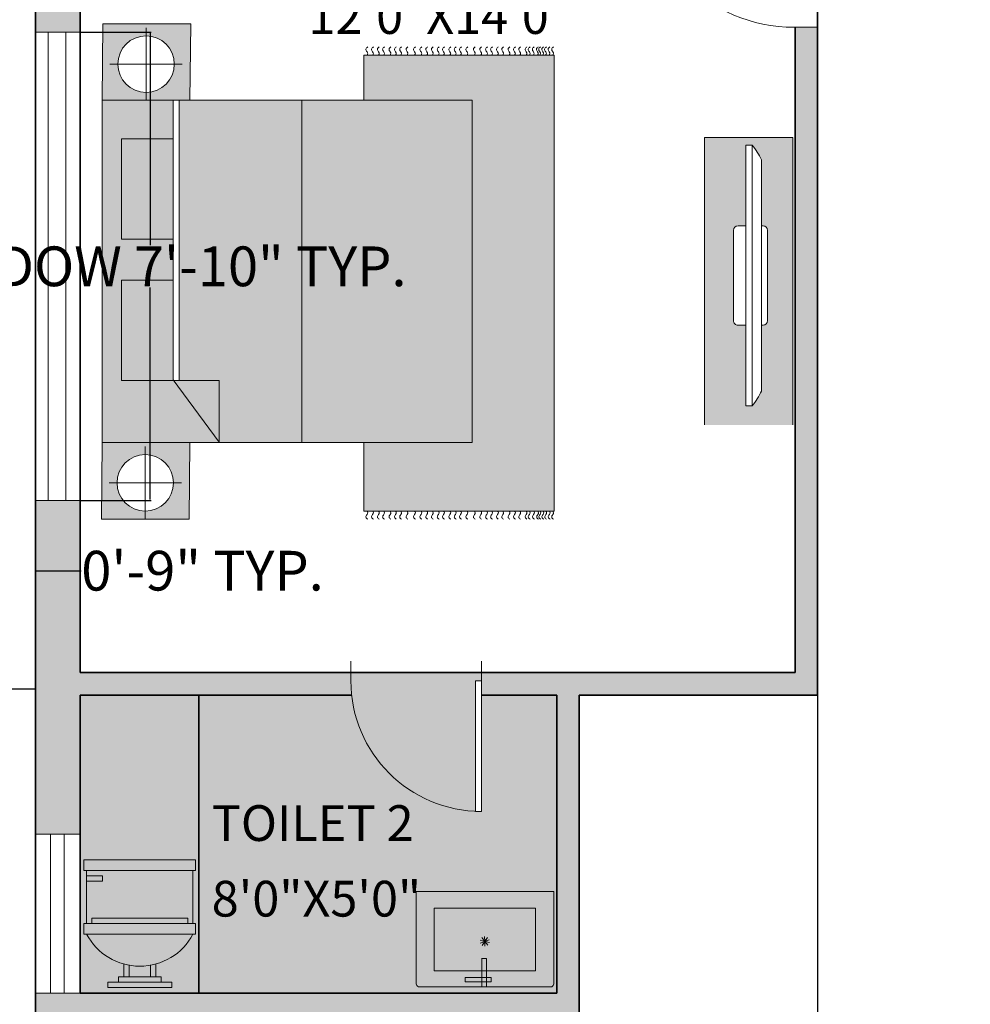
# Model space of a CAD drawing. Units: inches. Extents: x 853 to 1550, y 485 to 1596.
# Tile 4 of 18: x 979 to 1170, y 1010 to 1208. Entities that reach past the tile are written whole.
import ezdxf

# ---------------------------------------------------------------- set-up
doc = ezdxf.new("R2010")
doc.units = ezdxf.units.IN
doc.header["$MEASUREMENT"] = 0
for name, color, linetype, lineweight in [('A-ANNO-DIMS', 2, 'Continuous', 18), ('A-AREA-IDEN', 250, 'Continuous', 18), ('A-DOOR', 4, 'Continuous', 18), ('A-FLOR-CASE', 32, 'Continuous', 25), ('A-FLOR-FIXT', 8, 'Continuous', 18), ('A-WALL-PATT', 250, 'Continuous', 13), ('furniture', 250, 'Continuous', 18), ('walls', 250, 'Continuous', 35), ('windows', 4, 'Continuous', 18)]:
    doc.layers.add(name, color=color, linetype=linetype, lineweight=lineweight)
for name, color, linetype, lineweight, true_color in [('A-FIXT-PATT', 9, 'Continuous', 13, 0xc7c8ca), ('A-FLOR-TILE-PATT', 141, 'Continuous', 13, 0xadddf7), ('A-FURN-PATT', 254, 'Continuous', 13, 0xfeeab9)]:
    doc.layers.add(name, color=color, linetype=linetype, lineweight=lineweight, true_color=true_color)
doc.styles.get("Standard").update_dxf_attribs({"font": 'arial.ttf'})
doc.dimstyles.get("Standard").update_dxf_attribs({"dimtxt": 8, "dimasz": 0.18, "dimexe": 0.18, "dimexo": 0.0625, "dimgap": 0.09, "dimtad": 0, "dimtih": 1, "dimtoh": 1, "dimzin": 0, "dimdsep": 46, "dimlunit": 3, "dimtxsty": 'Standard', "dimcen": 0.09, "dimadec": 0, "dimazin": 0, "dimtfac": 1, "dimtofl": 0, "dimtmove": 0, "dimatfit": 3, "dimfxl": 1, "dimtolj": 1, "dimtzin": 0, "dimarcsym": 0})

# ---------------------------------------------------------------- blocks, each defined once
blk = doc.blocks.new('CARPET')
at = {"layer": 'furniture'}
for p, q in [((-51.53, -98.11), (-51.53, -55.12)), ((-51.53, -55.12), (-41.27, -55.12)), ((36, -55.12), (51.55, -55.12)), ((51.55, -55.12), (51.55, -98.11)), ((51.55, -98.11), (-51.53, -98.11))]:
    blk.add_line(p, q, dxfattribs=at)
for points, knots in [([(-53.37, -55.99), (-53.22, -55.8), (-52.9, -55.41), (-52.34, -55.8), (-51.89, -56.08), (-51.65, -55.91), (-51.53, -55.83)], [0, 0, 0, 0, 0.653278, 1.290138, 1.740457, 2.114451, 2.114451, 2.114451, 2.114451]), ([(53.37, -55.99), (53.22, -55.8), (52.9, -55.41), (52.34, -55.8), (51.89, -56.08), (51.65, -55.91), (51.53, -55.83)], [0, 0, 0, 0, 0.653278, 1.290138, 1.740457, 2.114451, 2.114451, 2.114451, 2.114451]), ([(-53.37, -57.26), (-53.22, -57.07), (-52.9, -56.67), (-52.34, -57.07), (-51.89, -57.35), (-51.65, -57.17), (-51.53, -57.1)], [0, 0, 0, 0, 0.653278, 1.290138, 1.740457, 2.114451, 2.114451, 2.114451, 2.114451]), ([(53.37, -57.26), (53.22, -57.07), (52.9, -56.67), (52.34, -57.07), (51.89, -57.35), (51.65, -57.17), (51.53, -57.1)], [0, 0, 0, 0, 0.653278, 1.290138, 1.740457, 2.114451, 2.114451, 2.114451, 2.114451]), ([(-53.37, -58.59), (-53.22, -58.4), (-52.9, -58.01), (-52.34, -58.4), (-51.89, -58.68), (-51.65, -58.5), (-51.53, -58.43)], [0, 0, 0, 0, 0.653278, 1.290138, 1.740457, 2.114451, 2.114451, 2.114451, 2.114451]), ([(-53.37, -59.78), (-53.22, -59.58), (-52.9, -59.19), (-52.34, -59.58), (-51.89, -59.86), (-51.65, -59.69), (-51.53, -59.61)], [0, 0, 0, 0, 0.653278, 1.290138, 1.740457, 2.114451, 2.114451, 2.114451, 2.114451]), ([(53.37, -58.59), (53.22, -58.4), (52.9, -58.01), (52.34, -58.4), (51.89, -58.68), (51.65, -58.5), (51.53, -58.43)], [0, 0, 0, 0, 0.653278, 1.290138, 1.740457, 2.114451, 2.114451, 2.114451, 2.114451]), ([(53.37, -59.78), (53.22, -59.58), (52.9, -59.19), (52.34, -59.58), (51.89, -59.86), (51.65, -59.69), (51.53, -59.61)], [0, 0, 0, 0, 0.653278, 1.290138, 1.740457, 2.114451, 2.114451, 2.114451, 2.114451]), ([(-53.37, -61.22), (-53.22, -61.02), (-52.9, -60.63), (-52.34, -61.02), (-51.89, -61.3), (-51.65, -61.13), (-51.53, -61.05)], [0, 0, 0, 0, 0.653278, 1.290138, 1.740457, 2.114451, 2.114451, 2.114451, 2.114451]), ([(-53.37, -62.44), (-53.22, -62.25), (-52.9, -61.86), (-52.34, -62.25), (-51.89, -62.53), (-51.65, -62.36), (-51.53, -62.28)], [0, 0, 0, 0, 0.653278, 1.290138, 1.740457, 2.114451, 2.114451, 2.114451, 2.114451]), ([(53.37, -61.22), (53.22, -61.02), (52.9, -60.63), (52.34, -61.02), (51.89, -61.3), (51.65, -61.13), (51.53, -61.05)], [0, 0, 0, 0, 0.653278, 1.290138, 1.740457, 2.114451, 2.114451, 2.114451, 2.114451]), ([(53.37, -62.44), (53.22, -62.25), (52.9, -61.86), (52.34, -62.25), (51.89, -62.53), (51.65, -62.36), (51.53, -62.28)], [0, 0, 0, 0, 0.653278, 1.290138, 1.740457, 2.114451, 2.114451, 2.114451, 2.114451]), ([(-53.37, -63.63), (-53.22, -63.43), (-52.9, -63.04), (-52.34, -63.43), (-51.89, -63.72), (-51.65, -63.54), (-51.53, -63.46)], [0, 0, 0, 0, 0.653278, 1.290138, 1.740457, 2.114451, 2.114451, 2.114451, 2.114451]), ([(53.37, -63.63), (53.22, -63.43), (52.9, -63.04), (52.34, -63.43), (51.89, -63.72), (51.65, -63.54), (51.53, -63.46)], [0, 0, 0, 0, 0.653278, 1.290138, 1.740457, 2.114451, 2.114451, 2.114451, 2.114451]), ([(-53.37, -65.07), (-53.22, -64.87), (-52.9, -64.48), (-52.34, -64.87), (-51.89, -65.15), (-51.65, -64.98), (-51.53, -64.9)], [0, 0, 0, 0, 0.653278, 1.290138, 1.740457, 2.114451, 2.114451, 2.114451, 2.114451]), ([(-53.37, -66.76), (-53.22, -66.56), (-52.9, -66.17), (-52.34, -66.56), (-51.89, -66.84), (-51.65, -66.67), (-51.53, -66.59)], [0, 0, 0, 0, 0.653278, 1.290138, 1.740457, 2.114451, 2.114451, 2.114451, 2.114451]), ([(53.37, -65.07), (53.22, -64.87), (52.9, -64.48), (52.34, -64.87), (51.89, -65.15), (51.65, -64.98), (51.53, -64.9)], [0, 0, 0, 0, 0.653278, 1.290138, 1.740457, 2.114451, 2.114451, 2.114451, 2.114451]), ([(53.37, -66.76), (53.22, -66.56), (52.9, -66.17), (52.34, -66.56), (51.89, -66.84), (51.65, -66.67), (51.53, -66.59)], [0, 0, 0, 0, 0.653278, 1.290138, 1.740457, 2.114451, 2.114451, 2.114451, 2.114451]), ([(-53.37, -68.2), (-53.22, -68), (-52.9, -67.61), (-52.34, -68), (-51.89, -68.28), (-51.65, -68.11), (-51.53, -68.03)], [0, 0, 0, 0, 0.653278, 1.290138, 1.740457, 2.114451, 2.114451, 2.114451, 2.114451]), ([(53.37, -68.2), (53.22, -68), (52.9, -67.61), (52.34, -68), (51.89, -68.28), (51.65, -68.11), (51.53, -68.03)], [0, 0, 0, 0, 0.653278, 1.290138, 1.740457, 2.114451, 2.114451, 2.114451, 2.114451]), ([(-53.37, -69.53), (-53.22, -69.33), (-52.9, -68.94), (-52.34, -69.33), (-51.89, -69.61), (-51.65, -69.44), (-51.53, -69.36)], [0, 0, 0, 0, 0.653278, 1.290138, 1.740457, 2.114451, 2.114451, 2.114451, 2.114451]), ([(-53.37, -70.79), (-53.22, -70.6), (-52.9, -70.21), (-52.34, -70.6), (-51.89, -70.88), (-51.65, -70.7), (-51.53, -70.63)], [0, 0, 0, 0, 0.653278, 1.290138, 1.740457, 2.114451, 2.114451, 2.114451, 2.114451]), ([(53.37, -69.53), (53.22, -69.33), (52.9, -68.94), (52.34, -69.33), (51.89, -69.61), (51.65, -69.44), (51.53, -69.36)], [0, 0, 0, 0, 0.653278, 1.290138, 1.740457, 2.114451, 2.114451, 2.114451, 2.114451]), ([(53.37, -70.79), (53.22, -70.6), (52.9, -70.21), (52.34, -70.6), (51.89, -70.88), (51.65, -70.7), (51.53, -70.63)], [0, 0, 0, 0, 0.653278, 1.290138, 1.740457, 2.114451, 2.114451, 2.114451, 2.114451]), ([(-53.37, -72.12), (-53.22, -71.93), (-52.9, -71.54), (-52.34, -71.93), (-51.89, -72.21), (-51.65, -72.04), (-51.53, -71.96)], [0, 0, 0, 0, 0.653278, 1.290138, 1.740457, 2.114451, 2.114451, 2.114451, 2.114451]), ([(-53.37, -73.31), (-53.22, -73.11), (-52.9, -72.72), (-52.34, -73.11), (-51.89, -73.4), (-51.65, -73.22), (-51.53, -73.14)], [0, 0, 0, 0, 0.653278, 1.290138, 1.740457, 2.114451, 2.114451, 2.114451, 2.114451]), ([(53.37, -72.12), (53.22, -71.93), (52.9, -71.54), (52.34, -71.93), (51.89, -72.21), (51.65, -72.04), (51.53, -71.96)], [0, 0, 0, 0, 0.653278, 1.290138, 1.740457, 2.114451, 2.114451, 2.114451, 2.114451]), ([(53.37, -73.31), (53.22, -73.11), (52.9, -72.72), (52.34, -73.11), (51.89, -73.4), (51.65, -73.22), (51.53, -73.14)], [0, 0, 0, 0, 0.653278, 1.290138, 1.740457, 2.114451, 2.114451, 2.114451, 2.114451]), ([(-53.37, -74.75), (-53.22, -74.55), (-52.9, -74.16), (-52.34, -74.55), (-51.89, -74.83), (-51.65, -74.66), (-51.53, -74.58)], [0, 0, 0, 0, 0.653278, 1.290138, 1.740457, 2.114451, 2.114451, 2.114451, 2.114451]), ([(-53.37, -75.98), (-53.22, -75.78), (-52.9, -75.39), (-52.34, -75.78), (-51.89, -76.06), (-51.65, -75.89), (-51.53, -75.81)], [0, 0, 0, 0, 0.653278, 1.290138, 1.740457, 2.114451, 2.114451, 2.114451, 2.114451]), ([(53.37, -74.75), (53.22, -74.55), (52.9, -74.16), (52.34, -74.55), (51.89, -74.83), (51.65, -74.66), (51.53, -74.58)], [0, 0, 0, 0, 0.653278, 1.290138, 1.740457, 2.114451, 2.114451, 2.114451, 2.114451]), ([(53.37, -75.98), (53.22, -75.78), (52.9, -75.39), (52.34, -75.78), (51.89, -76.06), (51.65, -75.89), (51.53, -75.81)], [0, 0, 0, 0, 0.653278, 1.290138, 1.740457, 2.114451, 2.114451, 2.114451, 2.114451]), ([(-53.37, -77.16), (-53.22, -76.96), (-52.9, -76.57), (-52.34, -76.96), (-51.89, -77.25), (-51.65, -77.07), (-51.53, -76.99)], [0, 0, 0, 0, 0.653278, 1.290138, 1.740457, 2.114451, 2.114451, 2.114451, 2.114451]), ([(53.37, -77.16), (53.22, -76.96), (52.9, -76.57), (52.34, -76.96), (51.89, -77.25), (51.65, -77.07), (51.53, -76.99)], [0, 0, 0, 0, 0.653278, 1.290138, 1.740457, 2.114451, 2.114451, 2.114451, 2.114451]), ([(-53.37, -78.6), (-53.22, -78.4), (-52.9, -78.01), (-52.34, -78.4), (-51.89, -78.68), (-51.65, -78.51), (-51.53, -78.43)], [0, 0, 0, 0, 0.653278, 1.290138, 1.740457, 2.114451, 2.114451, 2.114451, 2.114451]), ([(-53.37, -80.29), (-53.22, -80.09), (-52.9, -79.7), (-52.34, -80.09), (-51.89, -80.37), (-51.65, -80.2), (-51.53, -80.12)], [0, 0, 0, 0, 0.653278, 1.290138, 1.740457, 2.114451, 2.114451, 2.114451, 2.114451]), ([(53.37, -78.6), (53.22, -78.4), (52.9, -78.01), (52.34, -78.4), (51.89, -78.68), (51.65, -78.51), (51.53, -78.43)], [0, 0, 0, 0, 0.653278, 1.290138, 1.740457, 2.114451, 2.114451, 2.114451, 2.114451]), ([(53.37, -80.29), (53.22, -80.09), (52.9, -79.7), (52.34, -80.09), (51.89, -80.37), (51.65, -80.2), (51.53, -80.12)], [0, 0, 0, 0, 0.653278, 1.290138, 1.740457, 2.114451, 2.114451, 2.114451, 2.114451]), ([(-53.37, -81.73), (-53.22, -81.53), (-52.9, -81.14), (-52.34, -81.53), (-51.89, -81.81), (-51.65, -81.64), (-51.53, -81.56)], [0, 0, 0, 0, 0.653278, 1.290138, 1.740457, 2.114451, 2.114451, 2.114451, 2.114451]), ([(53.37, -81.73), (53.22, -81.53), (52.9, -81.14), (52.34, -81.53), (51.89, -81.81), (51.65, -81.64), (51.53, -81.56)], [0, 0, 0, 0, 0.653278, 1.290138, 1.740457, 2.114451, 2.114451, 2.114451, 2.114451]), ([(-53.37, -83.06), (-53.22, -82.86), (-52.9, -82.47), (-52.34, -82.86), (-51.89, -83.14), (-51.65, -82.97), (-51.53, -82.89)], [0, 0, 0, 0, 0.653278, 1.290138, 1.740457, 2.114451, 2.114451, 2.114451, 2.114451]), ([(-53.37, -84.18), (-53.22, -83.99), (-52.9, -83.6), (-52.34, -83.99), (-51.89, -84.27), (-51.65, -84.09), (-51.53, -84.02)], [0, 0, 0, 0, 0.653278, 1.290138, 1.740457, 2.114451, 2.114451, 2.114451, 2.114451]), ([(53.37, -83.06), (53.22, -82.86), (52.9, -82.47), (52.34, -82.86), (51.89, -83.14), (51.65, -82.97), (51.53, -82.89)], [0, 0, 0, 0, 0.653278, 1.290138, 1.740457, 2.114451, 2.114451, 2.114451, 2.114451]), ([(53.37, -84.18), (53.22, -83.99), (52.9, -83.6), (52.34, -83.99), (51.89, -84.27), (51.65, -84.09), (51.53, -84.02)], [0, 0, 0, 0, 0.653278, 1.290138, 1.740457, 2.114451, 2.114451, 2.114451, 2.114451]), ([(-53.37, -85.51), (-53.22, -85.32), (-52.9, -84.93), (-52.34, -85.32), (-51.89, -85.6), (-51.65, -85.42), (-51.53, -85.35)], [0, 0, 0, 0, 0.653278, 1.290138, 1.740457, 2.114451, 2.114451, 2.114451, 2.114451]), ([(-53.37, -86.7), (-53.22, -86.5), (-52.9, -86.11), (-52.34, -86.5), (-51.89, -86.78), (-51.65, -86.61), (-51.53, -86.53)], [0, 0, 0, 0, 0.653278, 1.290138, 1.740457, 2.114451, 2.114451, 2.114451, 2.114451]), ([(53.37, -85.51), (53.22, -85.32), (52.9, -84.93), (52.34, -85.32), (51.89, -85.6), (51.65, -85.42), (51.53, -85.35)], [0, 0, 0, 0, 0.653278, 1.290138, 1.740457, 2.114451, 2.114451, 2.114451, 2.114451]), ([(53.37, -86.7), (53.22, -86.5), (52.9, -86.11), (52.34, -86.5), (51.89, -86.78), (51.65, -86.61), (51.53, -86.53)], [0, 0, 0, 0, 0.653278, 1.290138, 1.740457, 2.114451, 2.114451, 2.114451, 2.114451]), ([(-53.37, -88.14), (-53.22, -87.94), (-52.9, -87.55), (-52.34, -87.94), (-51.89, -88.22), (-51.65, -88.05), (-51.53, -87.97)], [0, 0, 0, 0, 0.653278, 1.290138, 1.740457, 2.114451, 2.114451, 2.114451, 2.114451]), ([(-53.37, -89.36), (-53.22, -89.17), (-52.9, -88.78), (-52.34, -89.17), (-51.89, -89.45), (-51.65, -89.28), (-51.53, -89.2)], [0, 0, 0, 0, 0.653278, 1.290138, 1.740457, 2.114451, 2.114451, 2.114451, 2.114451]), ([(53.37, -88.14), (53.22, -87.94), (52.9, -87.55), (52.34, -87.94), (51.89, -88.22), (51.65, -88.05), (51.53, -87.97)], [0, 0, 0, 0, 0.653278, 1.290138, 1.740457, 2.114451, 2.114451, 2.114451, 2.114451]), ([(53.37, -89.36), (53.22, -89.17), (52.9, -88.78), (52.34, -89.17), (51.89, -89.45), (51.65, -89.28), (51.53, -89.2)], [0, 0, 0, 0, 0.653278, 1.290138, 1.740457, 2.114451, 2.114451, 2.114451, 2.114451]), ([(-53.37, -90.55), (-53.22, -90.35), (-52.9, -89.96), (-52.34, -90.35), (-51.89, -90.64), (-51.65, -90.46), (-51.53, -90.38)], [0, 0, 0, 0, 0.653278, 1.290138, 1.740457, 2.114451, 2.114451, 2.114451, 2.114451]), ([(53.37, -90.55), (53.22, -90.35), (52.9, -89.96), (52.34, -90.35), (51.9, -90.63), (51.66, -90.47), (51.55, -90.4)], [0, 0, 0, 0, 0.653278, 1.290138, 1.740457, 2.0926, 2.0926, 2.0926, 2.0926]), ([(-53.37, -91.99), (-53.22, -91.79), (-52.9, -91.4), (-52.34, -91.79), (-51.89, -92.07), (-51.65, -91.9), (-51.53, -91.82)], [0, 0, 0, 0, 0.653278, 1.290138, 1.740457, 2.114451, 2.114451, 2.114451, 2.114451]), ([(-53.37, -92.69), (-53.22, -92.48), (-52.9, -92.08), (-52.35, -92.49), (-51.89, -92.77), (-51.65, -92.6), (-51.53, -92.52)], [0, 0, 0, 0, 0.663904, 1.307406, 1.757725, 2.131719, 2.131719, 2.131719, 2.131719]), ([(-53.37, -93.61), (-53.22, -93.42), (-52.9, -93.03), (-52.34, -93.42), (-51.89, -93.7), (-51.65, -93.52), (-51.53, -93.45)], [0, 0, 0, 0, 0.653278, 1.290138, 1.740457, 2.114451, 2.114451, 2.114451, 2.114451]), ([(53.37, -91.99), (53.22, -91.79), (52.9, -91.4), (52.34, -91.79), (51.9, -92.07), (51.66, -91.91), (51.55, -91.83)], [0, 0, 0, 0, 0.653278, 1.290138, 1.740457, 2.0926, 2.0926, 2.0926, 2.0926]), ([(53.37, -92.69), (53.22, -92.49), (52.9, -92.09), (52.34, -92.49), (51.9, -92.77), (51.66, -92.61), (51.55, -92.53)], [0, 0, 0, 0, 0.656792, 1.295826, 1.746145, 2.098292, 2.098292, 2.098292, 2.098292]), ([(53.37, -93.66), (53.22, -93.46), (52.9, -93.07), (52.34, -93.46), (51.9, -93.74), (51.66, -93.58), (51.55, -93.5)], [0, 0, 0, 0, 0.653278, 1.290138, 1.740457, 2.0926, 2.0926, 2.0926, 2.0926]), ([(-53.37, -94.55), (-53.22, -94.35), (-52.9, -93.96), (-52.34, -94.35), (-51.89, -94.63), (-51.65, -94.46), (-51.53, -94.38)], [0, 0, 0, 0, 0.653278, 1.290138, 1.740457, 2.114451, 2.114451, 2.114451, 2.114451]), ([(-53.37, -95.05), (-53.22, -94.85), (-52.9, -94.46), (-52.34, -94.85), (-51.89, -95.14), (-51.65, -94.96), (-51.53, -94.88)], [0, 0, 0, 0, 0.653278, 1.290138, 1.740457, 2.114451, 2.114451, 2.114451, 2.114451]), ([(-53.37, -95.73), (-53.22, -95.54), (-52.9, -95.15), (-52.34, -95.54), (-51.89, -95.82), (-51.65, -95.65), (-51.53, -95.57)], [0, 0, 0, 0, 0.653278, 1.290138, 1.740457, 2.114451, 2.114451, 2.114451, 2.114451]), ([(53.37, -95.78), (53.22, -95.58), (52.9, -95.19), (52.34, -95.58), (51.89, -95.86), (51.65, -95.69), (51.53, -95.61)], [0, 0, 0, 0, 0.653278, 1.290138, 1.740457, 2.114451, 2.114451, 2.114451, 2.114451]), ([(53.37, -94.59), (53.22, -94.4), (52.9, -94.01), (52.34, -94.4), (51.9, -94.68), (51.66, -94.51), (51.55, -94.44)], [0, 0, 0, 0, 0.653278, 1.290138, 1.740457, 2.0926, 2.0926, 2.0926, 2.0926]), ([(53.37, -95.1), (53.22, -94.9), (52.9, -94.51), (52.34, -94.9), (51.9, -95.18), (51.66, -95.02), (51.55, -94.94)], [0, 0, 0, 0, 0.653278, 1.290138, 1.740457, 2.0926, 2.0926, 2.0926, 2.0926]), ([(-53.37, -96.38), (-53.22, -96.18), (-52.9, -95.79), (-52.34, -96.18), (-51.89, -96.47), (-51.65, -96.29), (-51.53, -96.21)], [0, 0, 0, 0, 0.653278, 1.290138, 1.740457, 2.114451, 2.114451, 2.114451, 2.114451]), ([(-53.37, -97.17), (-53.22, -96.98), (-52.9, -96.59), (-52.34, -96.98), (-51.89, -97.26), (-51.65, -97.08), (-51.53, -97.01)], [0, 0, 0, 0, 0.653278, 1.290138, 1.740457, 2.114451, 2.114451, 2.114451, 2.114451]), ([(-53.37, -97.99), (-53.22, -97.79), (-52.9, -97.4), (-52.34, -97.79), (-51.89, -98.08), (-51.65, -97.9), (-51.53, -97.82)], [0, 0, 0, 0, 0.653278, 1.290138, 1.740457, 2.114451, 2.114451, 2.114451, 2.114451]), ([(53.37, -96.43), (53.22, -96.23), (52.9, -95.84), (52.34, -96.23), (51.89, -96.51), (51.65, -96.34), (51.53, -96.26)], [0, 0, 0, 0, 0.653278, 1.290138, 1.740457, 2.114451, 2.114451, 2.114451, 2.114451]), ([(53.37, -97.22), (53.22, -97.02), (52.9, -96.63), (52.34, -97.02), (51.89, -97.3), (51.65, -97.13), (51.53, -97.05)], [0, 0, 0, 0, 0.653278, 1.290138, 1.740457, 2.114451, 2.114451, 2.114451, 2.114451]), ([(53.37, -97.99), (53.22, -97.79), (52.9, -97.4), (52.34, -97.79), (51.89, -98.08), (51.65, -97.9), (51.53, -97.82)], [0, 0, 0, 0, 0.653278, 1.290138, 1.740457, 2.114451, 2.114451, 2.114451, 2.114451])]:
    blk.add_open_spline(points, degree=3, knots=knots, dxfattribs=at)
blk = doc.blocks.new('A$C58D270C6')
at = {"layer": 'furniture'}
for p, q in [((9.09, 124.13), (9.09, 108.87)), ((1.46, 116.5), (16.73, 116.5)), ((14.97, 94.84), (24.62, 107.92)), ((24.62, 94.93), (24.62, 107.92)), ((42.08, 108), (42.08, 36)), ((14.97, 94.93), (24.62, 94.93)), ((14.97, 94.84), (14.97, 36)), ((16.22, 94.93), (16.22, 36)), ((9.25, 36), (9.25, 20.74)), ((1.62, 28.37), (16.88, 28.37))]:
    blk.add_line(p, q, dxfattribs=at)
for points in [[(18.5, 108), (18.34, 124.13), (-0.16, 124.13), (0, 108)], [(0, 108), (77.91, 108), (77.91, 36), (0, 36)], [(4.09, 94.93), (14.97, 94.93), (14.97, 73.83), (4.09, 73.83)], [(4.09, 65.23), (14.97, 65.23), (14.97, 44.13), (4.09, 44.13)], [(18.65, 19.87), (18.5, 36), (0, 36), (0.16, 19.87)]]:
    blk.add_lwpolyline(points, close=True, dxfattribs=at)
for centre in [(9.09, 116.5), (9.25, 28.37)]:
    blk.add_circle(centre, 5.95, dxfattribs=at)
at = {"layer": 'furniture', "xscale": 0.9312884925094044, "yscale": 0.9312884925094044, "zscale": 0.9312884925094044, "rotation": 90}
blk.add_blockref('CARPET', (3.79, 74.47), dxfattribs=at)
blk = doc.blocks.new('*U10')
for p, q in [((0, 0), (0, -6)), ((40, 0), (40, -6))]:
    blk.add_line(p, q)
blk.add_lwpolyline([(0, 0), (0, 40), (1.75, 40), (1.75, 0)], close=True)
blk.add_arc((0, 0), 40, 0, 90)
blk = doc.blocks.new('*U5')
for p, q in [((-10, 22), (-10, 12)), ((-10, 21), (-7, 21)), ((-7, 21), (-7, 20)), ((10, 12), (10, 22)), ((-7, 20), (-10, 20)), ((9, 13), (-9, 13)), ((-9, 13), (-9, 12)), ((9, 12), (9, 13)), ((10.5, 12), (-10.5, 12)), ((-10.5, 10), (-10.5, 12)), ((10.5, 12), (10.5, 10)), ((10.5, 10), (-10.5, 10)), ((-3, 4.4065), (-3, 2)), ((-2, 2), (-2, 4.1658)), ((2, 4.1658), (2, 2)), ((3, 2), (3, 4.4065)), ((4, 2), (-4, 2)), ((-4, 2), (-4, 1)), ((4, 1), (4, 2))]:
    blk.add_line(p, q)
for points in [[(10.5, 22), (10.5, 24), (-10.5, 24), (-10.5, 22)], [(6, 0), (6, 1), (-6, 1), (-6, 0)]]:
    blk.add_lwpolyline(points, close=True)
blk.add_arc((0, 15.3333), 11.3333, 208.0725, 331.9275)
blk = doc.blocks.new('*D21')
at = {"layer": 'A-ANNO-DIMS', "color": 0, "lineweight": -2, "transparency": 16777216}
for p, q in [((957.94, 1073.4), (957.94, 1073.52)), ((958.12, 1073.34), (966.1, 1073.34)), ((981.76, 1073.34), (973.78, 1073.34)), ((981.94, 1073.4), (981.94, 1073.52))]:
    blk.add_line(p, q, dxfattribs=at)
at = {"layer": 'A-ANNO-DIMS', "color": 0, "transparency": 16777216}
for points in [[(958.12, 1073.37), (958.12, 1073.31), (957.94, 1073.34)], [(981.76, 1073.37), (981.76, 1073.31), (981.94, 1073.34)]]:
    blk.add_solid(points, dxfattribs=at)
at = {"layer": 'Defpoints', "color": 0, "transparency": 16777216}
for p in [(957.94, 1073.34), (957.94, 1073.34), (981.94, 1073.34)]:
    blk.add_point(p, dxfattribs=at)
at = {"layer": 'A-ANNO-DIMS', "color": 0, "transparency": 16777216, "insert": (969.94, 1073.34), "char_height": 8, "attachment_point": 5}
blk.add_mtext("\\A1;2'", dxfattribs=at)
blk = doc.blocks.new('BASIN-RECT-WITH-MIXER')
for p, q in [((0, 3.21), (0, 19.18)), ((0, 19.18), (27.7, 19.18)), ((27.7, 19.18), (27.7, 0.61)), ((3.57, 3.21), (3.57, 15.84)), ((24, 15.84), (24, 3.21)), ((13.79, 9.14), (13.74, 10.1)), ((13.79, 9.14), (14.31, 9.95)), ((13.79, 9.14), (12.86, 9.39)), ((13.79, 9.14), (12.89, 8.8)), ((13.79, 9.14), (13.18, 9.89)), ((13.79, 9.14), (13.26, 8.33)), ((13.79, 9.14), (14.69, 9.48)), ((13.79, 9.14), (14.39, 8.39)), ((13.79, 9.14), (13.83, 8.18)), ((13.79, 9.14), (14.72, 8.89)), ((13.18, 5.79), (13.18, 0)), ((14.12, 5.69), (13.18, 5.69)), ((14.12, 0), (14.12, 5.69)), ((0, 0.61), (0, 3.21)), ((24, 3.21), (3.57, 3.21)), ((27.28, 0), (0.42, 0)), ((15.05, 1.84), (9.82, 1.84)), ((9.82, 1.84), (9.82, 0.98)), ((9.82, 0.98), (11.8, 0.98)), ((11.8, 0.98), (15.05, 0.98)), ((15.05, 0.98), (15.05, 1.84))]:
    blk.add_line(p, q)
for centre, start, end in [((0.76, 0.68), 185.6886, 243.8456), ((26.94, 0.68), 296.1544, 354.3114)]:
    blk.add_arc(centre, 0.761, start, end)
blk = doc.blocks.new('WIN-BATH-32IN')
for p, q in [((0, 32.01), (9, 32.01)), ((0, 0), (0, 32.01)), ((0, 32.01), (3.01, 32.01)), ((3.01, 32.01), (3.01, 0)), ((5.76, 0), (5.76, 32.01)), ((9, 32.01), (9, 0)), ((9, 0), (0, 0)), ((3.01, 0), (5.76, 0))]:
    blk.add_line(p, q)
blk = doc.blocks.new('WIN-94IN')
for p, q in [((0, 94.25), (9, 94.25)), ((0, 0), (0, 94.25)), ((2.54, 94.25), (2.54, 0)), ((6.1, 0), (6.1, 94.25)), ((9, 94.25), (9, 0)), ((9, 0), (0, 0)), ((2.54, 0), (6.1, 0))]:
    blk.add_line(p, q)
blk = doc.blocks.new('PLASMA-LARGE')
at = {"layer": 'furniture'}
for p, q in [((-7.26, 0), (7.26, 0)), ((-18.61, -1), (18.61, -1)), ((-8, -1), (-8, -0.74)), ((8, -1), (8, -0.74)), ((-21, -2.5), (21, -2.5)), ((-21, -2.5), (-21, -3.5)), ((21, -2.5), (21, -3.5)), ((-21, -3.5), (21, -3.5)), ((-8, -3.5), (-8, -4.76)), ((8, -3.5), (8, -4.76)), ((-7.26, -5.5), (7.26, -5.5))]:
    blk.add_line(p, q, dxfattribs=at)
for centre, radius, start, end in [((-7.26, -0.74), 0.744, 90, 180), ((7.26, -0.74), 0.744, 0, 90), ((-13.97, -11.05), 11.07, 114.7602, 129.4175), ((13.97, -11.05), 11.07, 50.5825, 65.2398), ((-7.26, -4.76), 0.744, 180, 270), ((7.26, -4.76), 0.744, 270, 0)]:
    blk.add_arc(centre, radius, start, end, dxfattribs=at)
blk = doc.blocks.new('TV-CONSOLE')
for p, q in [((0, 0), (0, 57.83)), ((0, 57.83), (17.81, 57.83)), ((17.81, 57.83), (17.81, 0))]:
    blk.add_line(p, q)
at = {"xscale": 1.249763490704796, "yscale": 1.249763490704796, "zscale": 1.249763490704796, "rotation": 270}
blk.add_blockref('PLASMA-LARGE', (12.71, 30.08), dxfattribs=at)
blk = doc.blocks.new('*D55')
at = {"layer": 'A-ANNO-DIMS', "color": 0, "lineweight": -2, "transparency": 16777216}
for p, q in [((991, 1205.54), (1005.25, 1205.54)), ((1005.07, 1205.36), (1005.07, 1162.64)), ((1005.07, 1111.47), (1005.07, 1154.18)), ((991, 1111.29), (1005.25, 1111.29))]:
    blk.add_line(p, q, dxfattribs=at)
at = {"layer": 'A-ANNO-DIMS', "color": 0, "transparency": 16777216}
for points in [[(1005.04, 1205.36), (1005.1, 1205.36), (1005.07, 1205.54)], [(1005.04, 1111.47), (1005.1, 1111.47), (1005.07, 1111.29)]]:
    blk.add_solid(points, dxfattribs=at)
at = {"layer": 'Defpoints', "color": 0, "transparency": 16777216}
for p in [(990.94, 1205.54), (1005.07, 1205.54), (990.94, 1111.29)]:
    blk.add_point(p, dxfattribs=at)
at = {"layer": 'A-ANNO-DIMS', "color": 0, "transparency": 16777216, "insert": (1005.07, 1158.41), "char_height": 8, "attachment_point": 5}
blk.add_mtext('\\A1;WINDOW 7\'-10" TYP.', dxfattribs=at)
blk = doc.blocks.new('*D56')
at = {"layer": 'A-ANNO-DIMS', "color": 0, "lineweight": -2, "transparency": 16777216}
for p, q in [((981.94, 1111.23), (981.94, 1096.97)), ((990.94, 1111.23), (990.94, 1096.97)), ((982.12, 1097.15), (990.76, 1097.15)), ((990.94, 1097.15), (991.12, 1097.15))]:
    blk.add_line(p, q, dxfattribs=at)
at = {"layer": 'A-ANNO-DIMS', "color": 0, "transparency": 16777216}
for points in [[(982.12, 1097.18), (982.12, 1097.12), (981.94, 1097.15)], [(990.76, 1097.18), (990.76, 1097.12), (990.94, 1097.15)]]:
    blk.add_solid(points, dxfattribs=at)
at = {"layer": 'Defpoints', "color": 0, "transparency": 16777216}
for p in [(981.94, 1111.29), (990.94, 1111.29), (990.94, 1097.15)]:
    blk.add_point(p, dxfattribs=at)
at = {"layer": 'A-ANNO-DIMS', "color": 0, "transparency": 16777216, "insert": (1015.59, 1097.15), "char_height": 8, "attachment_point": 5}
blk.add_mtext('\\A1;0\'-9" TYP.', dxfattribs=at)
blk = doc.blocks.new('*D65')
at = {"layer": 'A-ANNO-DIMS', "color": 0, "lineweight": -2, "transparency": 16777216}
for p, q in [((992.47, 993.79), (992.47, 997.14)), ((992.65, 996.96), (1013.89, 996.96)), ((1014.07, 993.79), (1014.07, 997.14)), ((1014.07, 996.96), (1014.25, 996.96))]:
    blk.add_line(p, q, dxfattribs=at)
at = {"layer": 'A-ANNO-DIMS', "color": 0, "transparency": 16777216}
for points in [[(992.65, 996.99), (992.65, 996.93), (992.47, 996.96)], [(1013.89, 996.99), (1013.89, 996.93), (1014.07, 996.96)]]:
    blk.add_solid(points, dxfattribs=at)
at = {"layer": 'Defpoints', "color": 0, "transparency": 16777216}
for p in [(1014.07, 996.96), (992.47, 993.72), (1014.07, 993.72)]:
    blk.add_point(p, dxfattribs=at)
at = {"layer": 'A-ANNO-DIMS', "color": 0, "transparency": 16777216, "insert": (1047.74, 996.96), "char_height": 8, "attachment_point": 5}
blk.add_mtext('\\A1;HOB 1\'-9 1/2"', dxfattribs=at)
blk = doc.blocks.new('*D70')
at = {"layer": 'A-ANNO-DIMS', "color": 0, "lineweight": -2, "transparency": 16777216}
for p, q in [((981.87, 1426.13), (877.09, 1426.13)), ((877.27, 1425.95), (877.27, 1067.22)), ((877.27, 700.05), (877.27, 1058.77)), ((1110.88, 699.87), (877.09, 699.87))]:
    blk.add_line(p, q, dxfattribs=at)
at = {"layer": 'A-ANNO-DIMS', "color": 0, "transparency": 16777216}
for points in [[(877.24, 1425.95), (877.3, 1425.95), (877.27, 1426.13)], [(877.24, 700.05), (877.3, 700.05), (877.27, 699.87)]]:
    blk.add_solid(points, dxfattribs=at)
at = {"layer": 'Defpoints', "color": 0, "transparency": 16777216}
for p in [(981.94, 1426.13), (877.27, 699.87), (1110.94, 699.87)]:
    blk.add_point(p, dxfattribs=at)
at = {"layer": 'A-ANNO-DIMS', "color": 0, "transparency": 16777216, "insert": (877.27, 1063), "char_height": 8, "attachment_point": 5}
blk.add_mtext('\\A1;60\'-6 1/2"', dxfattribs=at)
blk = doc.blocks.new('*D72')
at = {"layer": 'A-ANNO-DIMS', "color": 0, "lineweight": -2, "transparency": 16777216}
for p, q in [((1139.44, 1321.07), (1139.44, 497.1)), ((1199.44, 1321.07), (1199.44, 497.1)), ((1139.62, 497.28), (1158.71, 497.28)), ((1199.26, 497.28), (1180.16, 497.28))]:
    blk.add_line(p, q, dxfattribs=at)
at = {"layer": 'A-ANNO-DIMS', "color": 0, "transparency": 16777216}
for points in [[(1139.62, 497.31), (1139.62, 497.25), (1139.44, 497.28)], [(1199.26, 497.31), (1199.26, 497.25), (1199.44, 497.28)]]:
    blk.add_solid(points, dxfattribs=at)
at = {"layer": 'Defpoints', "color": 0, "transparency": 16777216}
for p in [(1139.44, 1321.13), (1199.44, 1321.13), (1199.44, 497.28)]:
    blk.add_point(p, dxfattribs=at)
at = {"layer": 'A-ANNO-DIMS', "color": 0, "transparency": 16777216, "insert": (1169.44, 497.28), "char_height": 8, "attachment_point": 5}
blk.add_mtext('\\A1;5\'-0"', dxfattribs=at)

msp = doc.modelspace()

# ---------------------------------------------------------------- hatches: boundary and pattern name
at = {"layer": 'A-FIXT-PATT'}
h = msp.add_hatch(color=256, dxfattribs=at)
h.dxf.hatch_style = 1
h.paths.add_polyline_path([(1013.667, 1036.821), (992.252, 1036.821), (992.252, 1035.751), (995.465, 1035.751), (995.465, 1034.68), (992.252, 1034.68), (992.252, 1026.114), (993.323, 1026.114), (993.323, 1027.185), (1012.596, 1027.185), (1012.596, 1026.114), (1013.667, 1026.114)])
h.paths.add_polyline_path([(1014.202, 1038.963), (991.717, 1038.963), (991.717, 1036.821), (1014.202, 1036.821)])
h.paths.add_polyline_path([(1014.202, 1026.114), (991.717, 1026.114), (991.717, 1023.973), (1014.202, 1023.973)])
h.paths.add_polyline_path([(1012.596, 1027.185), (993.323, 1027.185), (993.323, 1026.114), (1012.596, 1026.114)], flags=17)
h.paths.add_polyline_path([(1013.667, 1023.973), (992.252, 1023.973, 0.6000022)])
h.paths.add_polyline_path([(1000.818, 1017.739, -0.0226287), (999.748, 1017.981), (999.748, 1015.407), (1000.818, 1015.407)])
h.paths.add_polyline_path([(1006.172, 1017.981, -0.0226287), (1005.101, 1017.739), (1005.101, 1015.407), (1006.172, 1015.407)])
h.paths.add_polyline_path([(1007.243, 1015.407), (998.677, 1015.407), (998.677, 1014.336), (1007.243, 1014.336)])
h.paths.add_polyline_path([(1009.384, 1014.336), (996.535, 1014.336), (996.535, 1013.265), (1009.384, 1013.265)])
h = msp.add_hatch(color=256, dxfattribs=at)
h.dxf.hatch_style = 1
h.paths.add_polyline_path([(1062.202, 1029.244), (1082.638, 1029.244), (1082.638, 1016.616), (1072.752, 1016.616), (1072.752, 1015.245), (1073.687, 1015.245), (1073.687, 1014.386), (1072.752, 1014.386), (1072.752, 1013.408), (1085.909, 1013.408, 0.2593488), (1086.331, 1014.016), (1086.331, 1032.588), (1058.634, 1032.588), (1058.634, 1016.616), (1058.634, 1014.016, 0.2593488), (1059.056, 1013.408), (1071.816, 1013.408), (1071.816, 1014.386), (1070.433, 1014.386), (1068.45, 1014.386), (1068.45, 1015.245), (1071.816, 1015.245), (1071.816, 1016.616), (1062.202, 1016.616)])
h = msp.add_hatch(color=256, dxfattribs=at)
h.dxf.hatch_style = 1
h.paths.add_polyline_path([(1082.638, 1029.244), (1062.202, 1029.244), (1062.202, 1016.616), (1071.816, 1016.616), (1071.816, 1019.094), (1072.752, 1019.094), (1072.752, 1016.616), (1082.638, 1016.616)])
h.paths.add_polyline_path([(1074.446, 1022.548, -1), (1070.395, 1022.548, -1)], flags=16)
h.paths.add_polyline_path([(1073.383, 1022.548, -1), (1071.457, 1022.548, -1)], flags=0)
h.paths.add_polyline_path([(1072.752, 1019.094), (1071.816, 1019.094), (1071.816, 1016.616), (1072.752, 1016.616)], flags=17)
h.paths.add_polyline_path([(1072.752, 1016.616), (1071.816, 1016.616), (1071.816, 1015.245), (1072.752, 1015.245)])
h.paths.add_polyline_path([(1072.752, 1015.245), (1071.816, 1015.245), (1071.816, 1014.386), (1072.752, 1014.386)])
h.paths.add_polyline_path([(1071.816, 1015.245), (1068.45, 1015.245), (1068.45, 1014.386), (1070.433, 1014.386), (1071.816, 1014.386)])
h.paths.add_polyline_path([(1073.687, 1015.245), (1072.752, 1015.245), (1072.752, 1014.386), (1073.687, 1014.386)])
h.paths.add_polyline_path([(1072.752, 1014.386), (1071.816, 1014.386), (1071.816, 1013.408), (1072.752, 1013.408)])
h.paths.add_polyline_path([(1072.752, 1013.408), (1071.816, 1013.408), (1071.816, 1012.295), (1072.752, 1012.295)])
h = msp.add_hatch(color=256, dxfattribs=at)
h.dxf.hatch_style = 1
h.paths.add_polyline_path([(1070.395, 1022.548, 1), (1074.446, 1022.548, 1)])
h.paths.add_polyline_path([(1073.383, 1022.548, -1), (1071.457, 1022.548, -1)], flags=16)
at = {"layer": 'A-FLOR-TILE-PATT'}
h = msp.add_hatch(dxfattribs=at)
h.set_pattern_fill('ANGLE', color=256, scale=3)
h.set_pattern_definition([(0, (0, 0), (0, 0.825), [0.6, -0.225]), (90, (0, 0), (-0.825, 1e-16), [0.6, -0.225])])
h.paths.add_polyline_path([(1045.609, 1072.129), (1014.832, 1072.129), (1014.832, 1012.129), (1086.937, 1012.129), (1086.937, 1072.129), (1071.734, 1072.129), (1071.734, 1048.702), (1070.585, 1048.702), (1070.585, 1048.727, -0.3702014)])
h.paths.add_polyline_path([(1014.832, 1072.129), (990.937, 1072.129), (990.937, 1012.129), (1014.832, 1012.129)])
h.paths.add_polyline_path([(1070.585, 1074.983), (1071.734, 1074.983), (1071.734, 1076.629), (1045.453, 1076.629), (1045.453, 1074.983, 0.4014527), (1070.585, 1048.727)])
at = {"layer": 'A-FURN-PATT'}
h = msp.add_hatch(color=256, dxfattribs=at)
h.dxf.hatch_style = 1
h.paths.add_polyline_path([(1009.689, 1191.821), (995.368, 1191.821), (995.368, 1122.96), (1018.911, 1122.96), (1018.911, 1123.035), (1009.751, 1135.459), (999.283, 1135.459), (999.283, 1155.636), (1009.689, 1155.636), (1009.689, 1163.868), (999.283, 1163.868), (999.283, 1184.045), (1009.689, 1184.045)])
h.paths.add_polyline_path([(1018.911, 1135.459), (1009.751, 1135.459), (1018.911, 1123.035)], flags=17)
h.paths.add_polyline_path([(1009.76, 1114.831, -0.4142136), (1004.065, 1109.136), (1004.065, 1107.533), (1012.911, 1107.533), (1013.06, 1122.96), (995.368, 1122.96), (995.219, 1107.533), (1004.065, 1107.533), (1004.065, 1109.136, -0.4142136), (998.37, 1114.831, -1)])
h.paths.add_polyline_path([(1013.209, 1207.249), (995.516, 1207.249), (995.368, 1191.821), (1004.214, 1191.821), (1004.214, 1193.424, -0.4142136), (998.519, 1199.119, -1), (1009.909, 1199.119, -0.4142136), (1004.214, 1193.424), (1004.214, 1191.821), (1013.06, 1191.821)])
h = msp.add_hatch(color=256, dxfattribs=at)
h.dxf.hatch_style = 1
h.paths.add_polyline_path([(1086.377, 1200.926), (1048.091, 1200.926), (1048.091, 1191.821), (1069.876, 1191.821), (1069.876, 1122.96), (1048.091, 1122.96), (1048.091, 1109.108), (1086.377, 1109.108)])
h.paths.add_polyline_path([(1033.544, 1139.769), (1075.753, 1139.769), (1075.753, 1150.64), (1033.544, 1150.64)], flags=9)
h.paths.add_polyline_path([(1033.492, 1151.838), (1095.452, 1151.838), (1095.452, 1163.026), (1033.492, 1163.026)], flags=9)
h = msp.add_hatch(color=256, dxfattribs=at)
h.dxf.hatch_style = 1
h.paths.add_polyline_path([(1086.377, 1200.926), (1048.091, 1200.926), (1048.091, 1191.821), (1069.876, 1191.821), (1069.876, 1122.96), (1048.091, 1122.96), (1048.091, 1109.108), (1086.377, 1109.108)])
h = msp.add_hatch(color=256, dxfattribs=at)
h.dxf.hatch_style = 1
h.paths.add_polyline_path([(1069.876, 1191.821), (1035.611, 1191.821), (1035.611, 1122.96), (1069.876, 1122.96)])
h.paths.add_polyline_path([(1035.611, 1191.821), (1010.877, 1191.821), (1010.877, 1135.459), (1018.911, 1135.459), (1018.911, 1122.96), (1035.611, 1122.96)])
h = msp.add_hatch(color=256, dxfattribs=at)
h.dxf.hatch_style = 1
h.paths.add_polyline_path([(1009.689, 1155.636), (999.283, 1155.636), (999.283, 1135.459), (1009.689, 1135.459)])
h.paths.add_polyline_path([(1009.689, 1184.045), (999.283, 1184.045), (999.283, 1163.868), (1009.689, 1163.868)])
h = msp.add_hatch(color=256, dxfattribs=at)
h.dxf.hatch_style = 1
h.paths.add_polyline_path([(1116.674, 1184.324), (1116.674, 1126.49), (1134.486, 1126.49), (1134.486, 1184.324)])
h.paths.add_polyline_path([(1122.507, 1165.643, -0.4142136), (1123.437, 1166.573), (1125.006, 1166.573), (1125.006, 1182.82), (1126.256, 1182.82, -0.0640419), (1128.131, 1179.83), (1128.131, 1166.573), (1128.45, 1166.573, -0.4142136), (1129.381, 1165.643), (1129.381, 1147.507, -0.4142136), (1128.45, 1146.577), (1128.131, 1146.577), (1128.131, 1133.319, -0.0640419), (1126.256, 1130.33), (1125.006, 1130.33), (1125.006, 1146.577), (1123.437, 1146.577, -0.4142136), (1122.507, 1147.507)], flags=16)
at = {"layer": 'A-WALL-PATT'}
h = msp.add_hatch(color=256, dxfattribs=at)
h.dxf.hatch_style = 1
h.paths.add_polyline_path([(1139.437, 988.732), (1134.937, 988.732), (1134.937, 830.473), (1139.437, 830.473)])
h.paths.add_polyline_path([(1413.937, 1052.227), (1404.937, 1052.227), (1404.937, 1036.129), (1308.937, 1036.129), (1308.937, 1045.033), (1304.437, 1045.033), (1304.437, 1030.033), (1308.937, 1030.033), (1308.937, 1031.629), (1404.937, 1031.629), (1404.937, 863.629), (1365.241, 863.629), (1365.241, 854.629), (1413.937, 854.629)])
h.paths.add_polyline_path([(1413.937, 1133.918), (1404.937, 1133.918), (1404.937, 1100.629), (1304.437, 1100.629), (1304.437, 1078.26), (1308.937, 1078.26), (1308.937, 1096.129), (1404.937, 1096.129), (1404.937, 1084.233), (1407.946, 1084.233), (1413.937, 1084.233)])
h.paths.add_polyline_path([(1268.437, 1417.129), (1288.974, 1417.129), (1288.974, 1426.129), (1244.597, 1426.129), (1244.597, 1417.129), (1263.937, 1417.129), (1263.937, 1321.129), (1260.34, 1321.129), (1260.34, 1316.629), (1263.937, 1316.629), (1263.937, 1283.505), (1268.437, 1283.505)])
h.paths.add_polyline_path([(1413.937, 1426.129), (1360.402, 1426.129), (1360.402, 1417.129), (1404.937, 1417.129), (1404.937, 1249.129), (1268.437, 1249.129), (1268.437, 1254.041), (1268.357, 1254.041), (1263.937, 1254.041), (1263.937, 1244.629), (1404.937, 1244.629), (1404.937, 1228.163), (1413.937, 1228.163)])
h.paths.add_polyline_path([(1215.842, 1426.129), (1184.201, 1426.129), (1184.201, 1417.129), (1199.437, 1417.129), (1199.437, 1321.129), (1172.101, 1321.129), (1172.101, 1316.629), (1229.433, 1316.629), (1229.433, 1321.129), (1203.937, 1321.129), (1203.937, 1417.129), (1215.842, 1417.129)])
h.paths.add_polyline_path([(1139.437, 1417.129), (1155.446, 1417.129), (1155.446, 1426.129), (1091.831, 1426.129), (1091.831, 1417.129), (1134.937, 1417.129), (1134.937, 1289.22), (1139.437, 1289.22), (1139.437, 1316.629), (1143.553, 1316.629), (1143.553, 1321.129), (1139.437, 1321.129)])
h.paths.add_polyline_path([(1139.437, 1255.161), (1134.937, 1255.161), (1134.937, 1249.129), (990.937, 1249.129), (990.937, 1417.129), (1020.402, 1417.129), (1020.402, 1426.129), (981.937, 1426.129), (981.937, 1205.535), (984.477, 1205.535), (990.937, 1205.535), (990.937, 1244.629), (1134.937, 1244.629), (1134.937, 1237.775), (1139.437, 1237.775)])
h = msp.add_hatch(color=256, dxfattribs=at)
h.dxf.hatch_style = 1
h.paths.add_polyline_path([(990.937, 1111.29), (981.937, 1111.29), (981.937, 1044.136), (984.946, 1044.136), (990.937, 1044.136), (990.937, 1072.129), (1045.609, 1072.129, -0.0272078), (1045.453, 1074.983), (1045.453, 1076.629), (990.937, 1076.629)], flags=17)
h.paths.add_polyline_path([(1091.437, 1072.129), (1139.437, 1072.129), (1139.437, 1206.521), (1134.937, 1206.521), (1134.937, 1076.629), (1071.734, 1076.629), (1071.734, 1074.983), (1071.734, 1072.129), (1086.937, 1072.129), (1086.937, 1012.129), (990.937, 1012.129), (981.937, 1012.129), (981.937, 944.409), (990.937, 944.409), (990.937, 1007.629), (1091.437, 1007.629)])
h.paths.add_polyline_path([(990.937, 872.981), (981.937, 872.981), (981.937, 788.629), (990.937, 788.629)])
h.paths.add_polyline_path([(1014.605, 800.886), (990.937, 800.886), (990.937, 796.386), (1014.605, 796.386)])
h.paths.add_polyline_path([(1134.937, 793.129), (1090.727, 793.129), (1090.727, 788.629), (1134.937, 788.629)])
h.paths.add_polyline_path([(1139.437, 800.892), (1134.937, 800.892), (1134.937, 788.629), (1113.94, 788.629), (1113.94, 767.629), (1139.437, 767.629), (1191.938, 767.629), (1191.938, 772.657), (1191.938, 776.629), (1139.437, 776.629)])
h.paths.add_polyline_path([(1131.331, 781.621), (1131.331, 775.236), (1118.809, 775.236), (1118.809, 781.621)], flags=16)
h.paths.add_polyline_path([(1131.331, 781.621), (1118.809, 781.621), (1118.809, 775.236), (1131.331, 775.236)], flags=0)
h.paths.add_polyline_path([(1118.963, 707.356), (1110.94, 707.356), (1110.94, 699.868), (1118.963, 699.868)])
h.paths.add_polyline_path([(1284.919, 707.356), (1276.896, 707.356), (1276.896, 699.868), (1284.919, 699.868)])
h.paths.add_polyline_path([(1293.812, 863.629), (1268.437, 863.629), (1268.437, 984.936), (1308.937, 984.936), (1308.937, 996.627), (1304.437, 996.627), (1304.437, 989.436), (1263.937, 989.436), (1263.937, 863.629), (1215.364, 863.629), (1215.364, 854.629), (1252.179, 854.629), (1252.179, 776.629), (1225.216, 776.629, -0.0297134), (1225.453, 772.657), (1225.453, 767.629), (1261.179, 767.629), (1261.179, 854.629), (1293.812, 854.629)])
h.paths.add_polyline_path([(1176.151, 863.629), (1139.437, 863.629), (1139.437, 854.629), (1176.151, 854.629)])
h.paths.add_polyline_path([(1134.937, 863.629), (1109.834, 863.629), (1109.834, 859.129), (1134.937, 859.129)])
h.paths.add_polyline_path([(1148.879, 950.672), (1144.374, 950.672), (1144.374, 874.094), (1148.879, 874.094)])
h.paths.add_polyline_path([(1079.778, 863.629), (990.937, 863.629), (990.937, 859.129), (1079.778, 859.129)])

# ---------------------------------------------------------------- linework, layer by layer
at = {"layer": 'A-FLOR-CASE'}
for p, q in [((1014.832, 1072.129), (1014.832, 1012.129)), ((1014.832, 1012.129), (1014.832, 1072.129))]:
    msp.add_line(p, q, dxfattribs=at)
at = {"layer": 'A-FLOR-FIXT'}
msp.add_line((1062.202, 1029.244), (1082.638, 1029.244), dxfattribs=at)
at = {"layer": 'walls'}
for p, q in [((981.937, 788.629), (981.937, 1426.129)), ((1139.437, 1072.129), (1139.437, 1316.629)), ((990.937, 1076.629), (990.937, 1244.629)), ((1134.937, 1076.629), (1134.937, 1206.521)), ((990.937, 1076.629), (1134.937, 1076.629)), ((990.937, 1072.129), (1045.609, 1072.129)), ((990.937, 1012.129), (990.937, 1072.129)), ((1071.734, 1072.129), (1086.937, 1072.129)), ((1086.937, 1012.129), (1086.937, 1072.129)), ((1091.437, 1007.629), (1091.437, 1072.129)), ((1091.437, 1072.129), (1139.437, 1072.129)), ((990.937, 1012.129), (1086.937, 1012.129))]:
    msp.add_line(p, q, dxfattribs=at)
at = {"layer": 'windows'}
msp.add_line((981.937, 1205.535), (984.477, 1205.535), dxfattribs=at)

# ---------------------------------------------------------------- block references
at = {"layer": 'A-DOOR'}
for p, xscale, yscale, zscale, rotation in [((1134.749, 1237.775), -0.7813380285530513, 0.7813380285530513, 0.7813380285530513, 90), ((1071.734, 1074.983), 0.657032523498209, 0.657032523498209, 0.657032523498209, 180)]:
    msp.add_blockref('*U10', p, dxfattribs=dict(at, xscale=xscale, yscale=yscale, zscale=zscale, rotation=rotation))
at = {"layer": 'A-FLOR-FIXT', "xscale": 1.070727494090938, "yscale": 1.070727494090938, "zscale": 1.070727494090938}
msp.add_blockref('*U5', (1002.96, 1013.265), dxfattribs=at)
at = {"layer": 'A-FLOR-FIXT'}
msp.add_blockref('BASIN-RECT-WITH-MIXER', (1058.634, 1013.408), dxfattribs=at)
at = {"layer": 'furniture', "xscale": -0.9563987329230524, "yscale": 0.9563987329230524, "zscale": 0.9563987329230524, "rotation": 180}
msp.add_blockref('A$C58D270C6', (995.368, 1226.251), dxfattribs=at)
at = {"layer": 'furniture'}
msp.add_blockref('TV-CONSOLE', (1116.674, 1126.49), dxfattribs=at)
at = {"layer": 'windows'}
for name, p in [('WIN-94IN', (981.937, 1111.29)), ('WIN-BATH-32IN', (981.937, 1012.129))]:
    msp.add_blockref(name, p, dxfattribs=at)

# ---------------------------------------------------------------- texts
at = {"layer": 'A-AREA-IDEN'}
for s, height, p in [('12\'0"X14\'0"', 7.19435, (1036.907, 1205.188)), ('TOILET 2', 7.1944, (1017.432, 1042.756)), ('8\'0"X5\'0"', 7.1944, (1017.432, 1027.538))]:
    msp.add_text(s, height=height, dxfattribs=at).set_placement(p)

# ---------------------------------------------------------------- dimensions: what is measured, and where the dimension line sits
at = {"layer": 'A-ANNO-DIMS'}
dim = msp.add_linear_dim(base=(877.272, 699.868), p1=(981.937, 1426.129), p2=(1110.94, 699.868), angle=90, dimstyle='Standard', override={"dimdec": 1, "dimlfac": 1, "dimrnd": 0, "dimzin": 1, "dimdsep": 46, "dimlunit": 4, "dimfrac": 2}, dxfattribs=at)
dim.commit()
dim.dimension.update_dxf_attribs({"geometry": '*D70', "text_midpoint": (877.272, 1062.999)})
for base, p1, p2, override, picture, middle in [((1199.437, 497.279), (1139.437, 1321.129), (1199.437, 1321.129), {"dimdec": 1, "dimlfac": 1, "dimrnd": 0, "dimzin": 1, "dimdsep": 46, "dimlunit": 4, "dimfrac": 2}, '*D72', (1169.437, 497.279)), ((957.937, 1073.341), (981.937, 1073.341), (957.937, 1073.341), {"dimclrd": 0, "dimclre": 0, "dimclrt": 0}, '*D21', (969.937, 1073.341))]:
    dim = msp.add_linear_dim(base=base, p1=p1, p2=p2, dimstyle='Standard', override=override, dxfattribs=at)
    dim.commit()
    dim.dimension.update_dxf_attribs({"geometry": picture, "text_midpoint": middle})
dim = msp.add_linear_dim(base=(1005.074, 1205.535), p1=(990.937, 1111.29), p2=(990.937, 1205.535), angle=90, text='WINDOW <> TYP.', dimstyle='Standard', override={"dimdec": 1, "dimlfac": 1, "dimrnd": 0, "dimzin": 1, "dimdsep": 46, "dimlunit": 4, "dimfrac": 2}, dxfattribs=at)
dim.commit()
dim.dimension.update_dxf_attribs({"geometry": '*D55', "text_midpoint": (1005.074, 1158.413)})
for base, p1, p2, text, picture, middle in [((990.937, 1097.153), (981.937, 1111.29), (990.937, 1111.29), '<> TYP.', '*D56', (1015.589, 1097.153)), ((1014.071, 996.964), (992.471, 993.724), (1014.071, 993.724), 'HOB <>', '*D65', (1047.741, 996.964))]:
    dim = msp.add_linear_dim(base=base, p1=p1, p2=p2, text=text, dimstyle='Standard', override={"dimdec": 1, "dimlfac": 1, "dimrnd": 0, "dimzin": 1, "dimdsep": 46, "dimlunit": 4, "dimfrac": 2}, dxfattribs=at)
    dim.commit()
    dim.dimension.update_dxf_attribs({"geometry": picture, "text_midpoint": middle})

doc.saveas('drawing.dxf')
